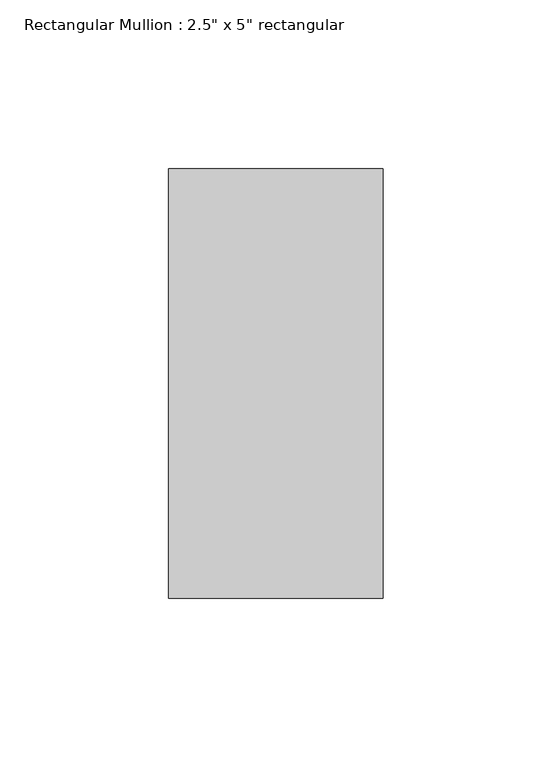
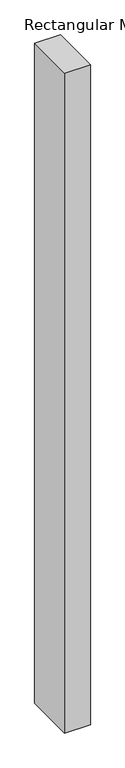
"""IFC4 building model written with IfcOpenShell, lengths in millimetres: member geometry."""

from ifc_helpers import new_model, si_unit, frame, origin, place, context, project, spatial, polyline, outline, extrude, source, transform, mapped, element, save


def member_3d200c31(model_context):
    return source(origin(), model_context, "Body", "SweptSolid", [
        extrude(outline(polyline([(31.75, 63.5), (31.75, -63.5), (-31.75, -63.5), (-31.75, 63.5), (31.75, 63.5)])), frame((0.0, 0.0, -1717.1019301), z_axis=(0.0, 0.0, 1.0), x_axis=(1.0, 0.0, 0.0)), (0.0, 0.0, 1.0), 1717.1019301),
    ])


if __name__ == "__main__":
    model = new_model("IFC4")
    model_context = context("Model", 3, world=origin())
    ifc_project = project(units=[si_unit("LENGTHUNIT", "METRE", prefix="MILLI")], contexts=[model_context])
    site = spatial("IfcSite", under=ifc_project)
    building = spatial("IfcBuilding", under=site)
    placement = place(None, origin())
    member_shape = member_3d200c31(model_context)
    element("IfcMember", 1, ObjectType="Rectangular Mullion : 2.5\" x 5\" rectangular", at=placement, inside=building, context=model_context, shape_type="MappedRepresentation", body=[
        mapped(member_shape, transform((0.0, 0.0, 0.0), x_axis=(1.0, 0.0, 0.0), y_axis=(0.0, 1.0, 0.0), z_axis=(0.0, 0.0, 1.0))),
    ])
    save(model, "model.ifc")

# Revit data of these elements
# Type "Rectangular Mullion : 2.5\" x 5\" rectangular"
#   built-in parameter 1007304 = 0.416667 (stored number, unit not read)
#   built-in parameter 1007301 = 0.104167 (stored number, unit not read)
#   built-in parameter 1007300 = 0.104167 (stored number, unit not read)
# Element 1 (IfcMember, "Rectangular Mullion : 2.5\" x 5\" rectangular")
#   Materials on its faces: "Aluminum"
# Materials
#   "Aluminum": class "Metal", colour RGB 247 247 247, transparency 0, Description = "Aluminum 6061", Cost = 0
